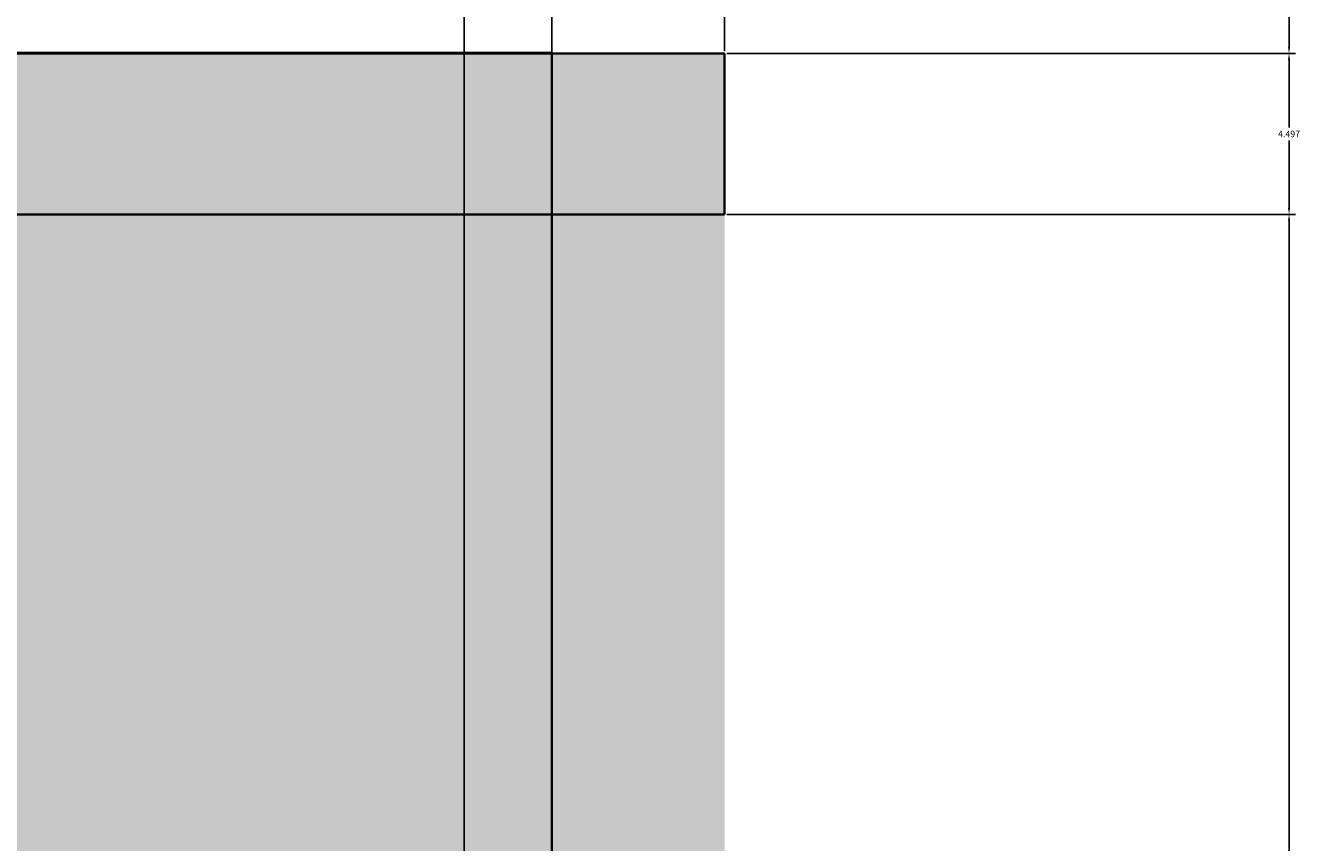
# Model space of a CAD drawing. Units: feet. Extents: x 2695 to 2912, y 795 to 1139.
# Tile 82 of 83: x 2876 to 2912, y 1086 to 1109. Entities that reach past the tile are written whole.
import ezdxf

# ---------------------------------------------------------------- set-up
doc = ezdxf.new("R2010")
doc.units = ezdxf.units.FT
for name, color, linetype, lineweight in [('A-ANNO-DIMS', 2, 'Continuous', 18), ('A-ELEV', 7, 'Continuous', 35), ('A-ELEV-PATT', 252, 'Continuous', 13)]:
    doc.layers.add(name, color=color, linetype=linetype, lineweight=lineweight)
doc.styles.get("Standard").update_dxf_attribs({"font": 'arial.ttf'})
doc.dimstyles.get("Standard").update_dxf_attribs({"dimtxt": 0.18, "dimasz": 0.18, "dimexe": 0.18, "dimexo": 0.0625, "dimgap": 0.09, "dimtad": 0, "dimtih": 1, "dimtoh": 1, "dimdec": 1, "dimzin": 0, "dimdsep": 46, "dimlunit": 3, "dimtxsty": 'Standard', "dimcen": 0.09, "dimadec": 0, "dimazin": 0, "dimtfac": 1, "dimtdec": 1, "dimtofl": 0, "dimtmove": 0, "dimatfit": 3, "dimfxl": 1, "dimtolj": 1, "dimtzin": 0, "dimarcsym": 0})

# ---------------------------------------------------------------- blocks, each defined once
blk = doc.blocks.new('*D11')
at = {"layer": 'A-ANNO-DIMS', "color": 0, "lineweight": -2, "transparency": 16777216}
for p, q in [((2843.575, 1020.886), (2843.575, 1138.886)), ((2843.755, 1138.706), (2869.128, 1138.706)), ((2895.289, 1138.706), (2869.916, 1138.706)), ((2895.469, 1107.898), (2895.469, 1138.886))]:
    blk.add_line(p, q, dxfattribs=at)
at = {"layer": 'A-ANNO-DIMS', "color": 0, "transparency": 16777216}
for points in [[(2843.755, 1138.736), (2843.755, 1138.676), (2843.575, 1138.706)], [(2895.289, 1138.736), (2895.289, 1138.676), (2895.469, 1138.706)]]:
    blk.add_solid(points, dxfattribs=at)
at = {"layer": 'Defpoints', "color": 0, "transparency": 16777216}
for p in [(2895.469, 1138.706), (2895.469, 1107.835), (2843.575, 1020.824)]:
    blk.add_point(p, dxfattribs=at)
at = {"layer": 'A-ANNO-DIMS', "color": 0, "transparency": 16777216, "insert": (2869.522, 1138.706), "char_height": 0.18, "attachment_point": 5}
blk.add_mtext('\\A1;51.89', dxfattribs=at)
blk = doc.blocks.new('*D20')
at = {"layer": 'A-ANNO-DIMS', "color": 0, "lineweight": -2, "transparency": 16777216}
for p, q in [((2895.532, 1103.338), (2911.424, 1103.338)), ((2911.244, 1103.158), (2911.244, 1083.316)), ((2911.244, 1063.111), (2911.244, 1082.952)), ((2890.699, 1062.931), (2911.424, 1062.931))]:
    blk.add_line(p, q, dxfattribs=at)
at = {"layer": 'A-ANNO-DIMS', "color": 0, "transparency": 16777216}
for points in [[(2911.214, 1103.158), (2911.274, 1103.158), (2911.244, 1103.338)], [(2911.214, 1063.111), (2911.274, 1063.111), (2911.244, 1062.931)]]:
    blk.add_solid(points, dxfattribs=at)
at = {"layer": 'Defpoints', "color": 0, "transparency": 16777216}
for p in [(2895.469, 1103.338), (2911.244, 1103.338), (2890.636, 1062.931)]:
    blk.add_point(p, dxfattribs=at)
at = {"layer": 'A-ANNO-DIMS', "color": 0, "transparency": 16777216, "insert": (2911.244, 1083.134), "char_height": 0.18, "attachment_point": 5}
blk.add_mtext('\\A1;40.41', dxfattribs=at)
blk = doc.blocks.new('*D21')
at = {"layer": 'A-ANNO-DIMS', "color": 0, "lineweight": -2, "transparency": 16777216}
for p, q in [((2895.532, 1107.835), (2911.424, 1107.835)), ((2911.244, 1107.655), (2911.244, 1105.768)), ((2911.244, 1103.518), (2911.244, 1105.405)), ((2895.532, 1103.338), (2911.424, 1103.338))]:
    blk.add_line(p, q, dxfattribs=at)
at = {"layer": 'A-ANNO-DIMS', "color": 0, "transparency": 16777216}
for points in [[(2911.214, 1107.655), (2911.274, 1107.655), (2911.244, 1107.835)], [(2911.214, 1103.518), (2911.274, 1103.518), (2911.244, 1103.338)]]:
    blk.add_solid(points, dxfattribs=at)
at = {"layer": 'Defpoints', "color": 0, "transparency": 16777216}
for p in [(2895.469, 1107.835), (2911.244, 1107.835), (2895.469, 1103.338)]:
    blk.add_point(p, dxfattribs=at)
at = {"layer": 'A-ANNO-DIMS', "color": 0, "transparency": 16777216, "insert": (2911.244, 1105.586), "char_height": 0.18, "attachment_point": 5}
blk.add_mtext('\\A1;4.497', dxfattribs=at)
blk = doc.blocks.new('*D22')
at = {"layer": 'A-ANNO-DIMS', "color": 0, "lineweight": -2, "transparency": 16777216}
for p, q in [((2770.699, 1122.931), (2911.424, 1122.931)), ((2911.244, 1122.751), (2911.244, 1115.565)), ((2911.244, 1108.015), (2911.244, 1115.201)), ((2895.532, 1107.835), (2911.424, 1107.835))]:
    blk.add_line(p, q, dxfattribs=at)
at = {"layer": 'A-ANNO-DIMS', "color": 0, "transparency": 16777216}
for points in [[(2911.214, 1122.751), (2911.274, 1122.751), (2911.244, 1122.931)], [(2911.214, 1108.015), (2911.274, 1108.015), (2911.244, 1107.835)]]:
    blk.add_solid(points, dxfattribs=at)
at = {"layer": 'Defpoints', "color": 0, "transparency": 16777216}
for p in [(2770.636, 1122.931), (2911.244, 1122.931), (2895.469, 1107.835)]:
    blk.add_point(p, dxfattribs=at)
at = {"layer": 'A-ANNO-DIMS', "color": 0, "transparency": 16777216, "insert": (2911.244, 1115.383), "char_height": 0.18, "attachment_point": 5}
blk.add_mtext('\\A1;15.095', dxfattribs=at)
blk = doc.blocks.new('*D50')
at = {"layer": 'A-ANNO-DIMS', "color": 0, "lineweight": -2, "transparency": 16777216}
for p, q in [((2810.041, 972.03), (2810.041, 1138.886)), ((2810.221, 1138.706), (2848.721, 1138.706)), ((2888.008, 1138.706), (2849.508, 1138.706)), ((2888.188, 972.03), (2888.188, 1138.886))]:
    blk.add_line(p, q, dxfattribs=at)
at = {"layer": 'A-ANNO-DIMS', "color": 0, "transparency": 16777216}
for points in [[(2810.221, 1138.736), (2810.221, 1138.676), (2810.041, 1138.706)], [(2888.008, 1138.736), (2888.008, 1138.676), (2888.188, 1138.706)]]:
    blk.add_solid(points, dxfattribs=at)
at = {"layer": 'Defpoints', "color": 0, "transparency": 16777216}
for p in [(2888.188, 1138.706), (2810.041, 971.967), (2888.188, 971.967)]:
    blk.add_point(p, dxfattribs=at)
at = {"layer": 'A-ANNO-DIMS', "color": 0, "transparency": 16777216, "insert": (2849.114, 1138.706), "char_height": 0.18, "attachment_point": 5}
blk.add_mtext('\\A1;78.15', dxfattribs=at)
blk = doc.blocks.new('*D51')
at = {"layer": 'A-ANNO-DIMS', "color": 0, "lineweight": -2, "transparency": 16777216}
for p, q in [((2888.188, 972.03), (2888.188, 1138.886)), ((2888.368, 1138.706), (2889.017, 1138.706)), ((2890.456, 1138.706), (2889.808, 1138.706)), ((2890.636, 972.03), (2890.636, 1138.886))]:
    blk.add_line(p, q, dxfattribs=at)
at = {"layer": 'A-ANNO-DIMS', "color": 0, "transparency": 16777216}
for points in [[(2888.368, 1138.736), (2888.368, 1138.676), (2888.188, 1138.706)], [(2890.456, 1138.736), (2890.456, 1138.676), (2890.636, 1138.706)]]:
    blk.add_solid(points, dxfattribs=at)
at = {"layer": 'Defpoints', "color": 0, "transparency": 16777216}
for p in [(2890.636, 1138.706), (2888.188, 971.967), (2890.636, 971.967)]:
    blk.add_point(p, dxfattribs=at)
at = {"layer": 'A-ANNO-DIMS', "color": 0, "transparency": 16777216, "insert": (2889.412, 1138.706), "char_height": 0.18, "attachment_point": 5}
blk.add_mtext('\\A1;2.448', dxfattribs=at)

msp = doc.modelspace()

# ---------------------------------------------------------------- hatches: boundary and pattern name
at = {"layer": 'A-ELEV-PATT'}
h = msp.add_hatch(color=256, dxfattribs=at)
h.set_gradient(color1=(255, 255, 255), tint=1)
h.paths.add_polyline_path([(2770.6361, 1122.9306), (2710.6361, 1122.9306), (2710.6361, 1118.4096), (2770.6361, 1118.4096)])
h.paths.add_polyline_path([(2890.6361, 1107.8588), (2770.6361, 1107.8588), (2770.6361, 1103.3378), (2890.6361, 1103.3378)])
h.paths.add_polyline_path([(2890.6361, 1062.9306), (2710.6361, 1062.9306), (2710.6361, 1056.9306), (2710.6361, 936.9306), (2710.6361, 924.3105), (2716.5358, 924.3105), (2890.6361, 924.3105), (2890.6361, 936.9306), (2715.8852, 936.9306), (2715.8852, 1050.3105), (2890.6361, 1050.3105)])
h.paths.add_polyline_path([(2716.5358, 924.3105), (2710.6361, 924.3105), (2710.6361, 810.9306), (2716.5358, 810.9306)])
h = msp.add_hatch(color=256, dxfattribs=at)
h.set_gradient(color1=(147, 149, 152), color2=(147, 149, 152), tint=1)
h.paths.add_polyline_path([(2770.6361, 1118.4096), (2710.6361, 1118.4096), (2710.6361, 1062.9306), (2770.6361, 1062.9306)])
h.paths.add_polyline_path([(2890.6361, 1103.3378), (2770.6361, 1103.3378), (2770.6361, 1062.9306), (2890.6361, 1062.9306)])
h.paths.add_polyline_path([(2730.7081, 1048.1052), (2755.1125, 1048.1052), (2755.1125, 936.9306), (2770.6361, 936.9306), (2770.6361, 1050.3105), (2715.8852, 1050.3105), (2715.8852, 936.9306), (2730.7081, 936.9306)])
h.paths.add_polyline_path([(2890.6361, 1050.3105), (2770.6361, 1050.3105), (2770.6361, 971.9673), (2778.0341, 971.9673), (2778.0341, 1020.8235), (2843.575, 1020.8235), (2843.575, 971.9673), (2890.6361, 971.9673)])
h.paths.add_polyline_path([(2888.1882, 970.7156), (2843.575, 970.7156), (2843.575, 964.8267), (2888.1882, 964.8267)])
h.paths.add_polyline_path([(2888.1882, 964.1328), (2843.575, 964.1328), (2843.575, 956.614), (2888.1882, 956.614)])
h.paths.add_polyline_path([(2888.1882, 955.9202), (2843.575, 955.9202), (2843.575, 949.2892), (2888.1882, 949.2892)])
h.paths.add_polyline_path([(2888.1882, 948.5954), (2843.575, 948.5954), (2843.575, 941.3507), (2888.1882, 941.3507)])
h.paths.add_polyline_path([(2888.1882, 940.6569), (2843.575, 940.6569), (2843.575, 936.9306), (2888.1882, 936.9306)])
h.paths.add_polyline_path([(2890.6361, 970.7156), (2888.9368, 970.7156), (2888.9368, 964.8267), (2890.6361, 964.8267)])
h.paths.add_polyline_path([(2890.6361, 964.1328), (2888.9368, 964.1328), (2888.9368, 956.614), (2890.6361, 956.614)])
h.paths.add_polyline_path([(2890.6361, 955.9202), (2888.9368, 955.9202), (2888.9368, 949.2892), (2890.6361, 949.2892)])
h.paths.add_polyline_path([(2890.6361, 940.6569), (2888.9368, 940.6569), (2888.9368, 936.9306), (2890.6361, 936.9306)])
h.paths.add_polyline_path([(2890.6361, 948.5954), (2888.9368, 948.5954), (2888.9368, 941.3507), (2890.6361, 941.3507)])
h.paths.add_polyline_path([(2772.5216, 970.7156), (2770.6361, 970.7156), (2770.6361, 964.8267), (2772.5216, 964.8267)])
h.paths.add_polyline_path([(2772.5216, 964.1328), (2770.6361, 964.1328), (2770.6361, 956.614), (2772.5216, 956.614)])
h.paths.add_polyline_path([(2772.5216, 955.9202), (2770.6361, 955.9202), (2770.6361, 949.2892), (2772.5216, 949.2892)])
h.paths.add_polyline_path([(2772.5216, 948.5954), (2770.6361, 948.5954), (2770.6361, 941.3507), (2772.5216, 941.3507)])
h.paths.add_polyline_path([(2772.5216, 940.6569), (2770.6361, 940.6569), (2770.6361, 936.9306), (2772.5216, 936.9306)])
h.paths.add_polyline_path([(2778.0341, 940.6569), (2773.2702, 940.6569), (2773.2702, 936.9306), (2778.0341, 936.9306)])
h.paths.add_polyline_path([(2778.0341, 970.7156), (2773.2702, 970.7156), (2773.2702, 964.8267), (2778.0341, 964.8267)])
h.paths.add_polyline_path([(2778.0341, 964.1328), (2773.2702, 964.1328), (2773.2702, 956.614), (2778.0341, 956.614)])
h.paths.add_polyline_path([(2778.0341, 955.9202), (2773.2702, 955.9202), (2773.2702, 949.2892), (2778.0341, 949.2892)])
h.paths.add_polyline_path([(2778.0341, 948.5954), (2773.2702, 948.5954), (2773.2702, 941.3507), (2778.0341, 941.3507)])
h.paths.add_polyline_path([(2810.0407, 940.6569), (2780.0341, 940.6569), (2780.0341, 936.9306), (2810.0407, 936.9306)])
h.paths.add_polyline_path([(2890.6361, 924.3105), (2770.6361, 924.3105), (2770.6361, 810.9306), (2773.5029, 810.9306), (2773.5029, 905.5143), (2805.9398, 905.5143), (2838.3767, 905.5143), (2838.3767, 810.9306), (2890.6361, 810.9306)])
h = msp.add_hatch(color=256, dxfattribs=at)
h.set_gradient(color1=(255, 255, 255), tint=1)
h.paths.add_polyline_path([(2895.4694, 1107.8588), (2890.6361, 1107.8588), (2890.6361, 810.9306), (2895.4694, 810.9306)])
h = msp.add_hatch(color=256, dxfattribs=at)
h.set_gradient(color1=(199, 200, 202), color2=(213, 227, 240), centered=1)
h.paths.add_polyline_path([(2890.6361, 1103.3378), (2770.6361, 1103.3378), (2770.6361, 1062.9306), (2890.6361, 1062.9306)])
h = msp.add_hatch(color=256, dxfattribs=at)
h.set_gradient(color1=(147, 149, 152), color2=(147, 149, 152), tint=1)
h.paths.add_polyline_path([(2895.4694, 1103.3378), (2890.6361, 1103.3378), (2890.6361, 1062.9306), (2895.4694, 1062.9306)])

# ---------------------------------------------------------------- linework, layer by layer
at = {"layer": 'A-ELEV'}
for p, q in [((2770.6361, 1107.8588), (2890.6361, 1107.8588)), ((2895.4694, 1107.8352), (2770.6361, 1107.8588)), ((2890.6361, 810.9306), (2890.6361, 1107.8588)), ((2895.4694, 1103.3378), (2895.4694, 1107.8352)), ((2770.6361, 1103.3378), (2895.4694, 1103.3378)), ((2890.6361, 1103.3378), (2895.4694, 1103.3378))]:
    msp.add_line(p, q, dxfattribs=at)
msp.add_lwpolyline([(2770.6361, 1103.3378), (2890.6361, 1103.3378)], dxfattribs=at)

# ---------------------------------------------------------------- dimensions: what is measured, and where the dimension line sits
at = {"layer": 'A-ANNO-DIMS'}
for base, p1, p2, override, picture, middle in [((2888.1882, 1138.7056), (2810.0407, 971.9673), (2888.1882, 971.9673), {"dimdec": 2, "dimlfac": 1, "dimrnd": 0, "dimzin": 0, "dimdsep": 46, "dimlunit": 2}, '*D50', (2849.1144, 1138.7056)), ((2895.4694, 1138.7056), (2843.575, 1020.8235), (2895.4694, 1107.8352), {"dimdec": 2, "dimlfac": 1, "dimrnd": 0, "dimzin": 0, "dimdsep": 46, "dimlunit": 2}, '*D11', (2869.5222, 1138.7056)), ((2890.6361, 1138.7056), (2888.1882, 971.9673), (2890.6361, 971.9673), {"dimdec": 3, "dimlfac": 1, "dimrnd": 0, "dimzin": 0, "dimdsep": 46, "dimlunit": 2}, '*D51', (2889.4121, 1138.7056))]:
    dim = msp.add_linear_dim(base=base, p1=p1, p2=p2, dimstyle='Standard', override=override, dxfattribs=at)
    dim.commit()
    dim.dimension.update_dxf_attribs({"geometry": picture, "text_midpoint": middle})
for base, p1, p2, override, picture, middle in [((2911.2444, 1122.9306), (2895.4694, 1107.8352), (2770.6361, 1122.9306), {"dimdec": 3, "dimlfac": 1, "dimrnd": 0, "dimzin": 0, "dimdsep": 46, "dimlunit": 2}, '*D22', (2911.2444, 1115.3829)), ((2911.2444, 1107.8352), (2895.4694, 1103.3378), (2895.4694, 1107.8352), {"dimdec": 3, "dimlfac": 1, "dimrnd": 0, "dimzin": 0, "dimdsep": 46, "dimlunit": 2}, '*D21', (2911.2444, 1105.5865)), ((2911.2444, 1103.3378), (2890.6361, 1062.9306), (2895.4694, 1103.3378), {"dimdec": 2, "dimlfac": 1, "dimrnd": 0, "dimzin": 0, "dimdsep": 46, "dimlunit": 2}, '*D20', (2911.2444, 1083.1342))]:
    dim = msp.add_linear_dim(base=base, p1=p1, p2=p2, angle=90, dimstyle='Standard', override=override, dxfattribs=at)
    dim.commit()
    dim.dimension.update_dxf_attribs({"geometry": picture, "text_midpoint": middle})

doc.saveas('drawing.dxf')
